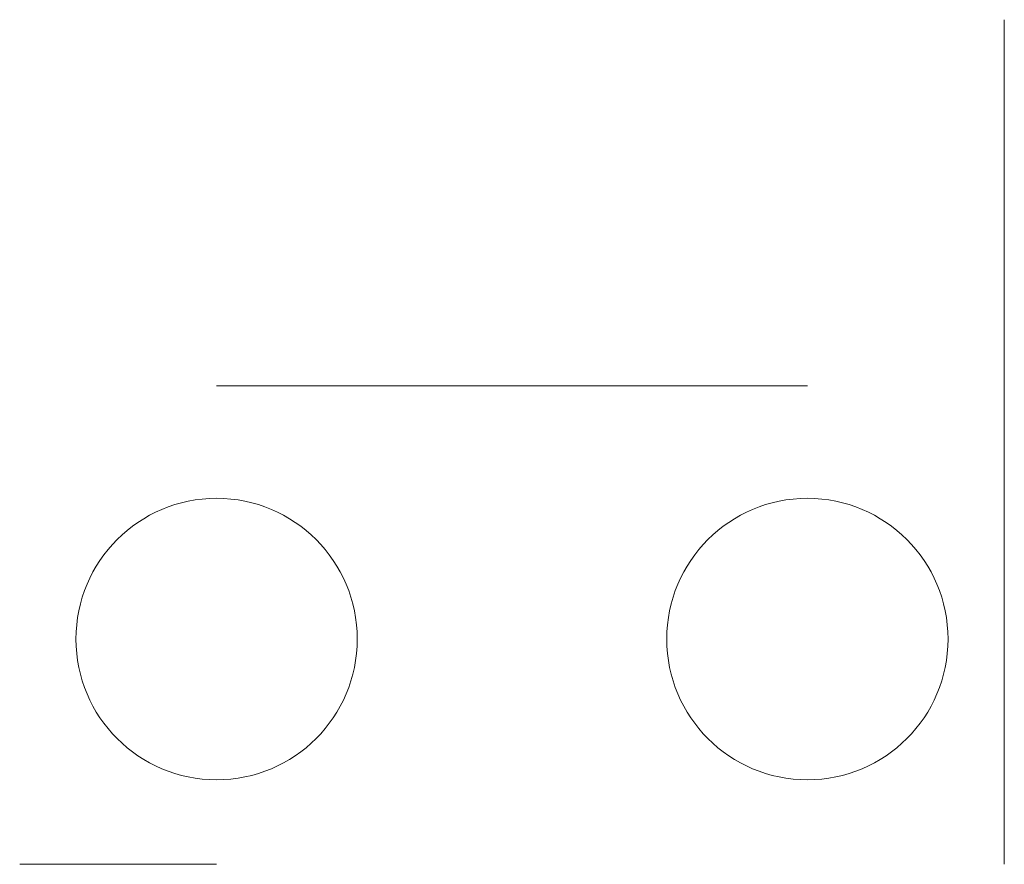
# Model space of a CAD drawing. Units: millimetres. Extents: x -35 to 77, y -482 to 0.
# Tile 1 of 2: x -35 to 0, y -482 to -452. Entities that reach past the tile are written whole.
import ezdxf

# ---------------------------------------------------------------- set-up
doc = ezdxf.new("R2010")
doc.units = ezdxf.units.MM
doc.layers.add('M-CONS', color=8, linetype='Continuous', lineweight=13)

msp = doc.modelspace()

# ---------------------------------------------------------------- linework, layer by layer
at = {"layer": 'M-CONS', "extrusion": (-1, 0, 0)}
for p, q in [((0, -452.364, 152.362), (0, -482.364, 152.362)), ((0, -452.364, 222.362), (0, -452.364, 152.362)), ((0, -460.364, 227.362), (0, -457.364, 227.362)), ((0, -482.364, 162.362), (0, -459.364, 162.362)), ((0, -459.364, 162.362), (0, -459.364, 207.362)), ((0, -459.364, 207.362), (0, -465.364, 207.362)), ((0, -465.364, 207.362), (0, -465.364, 222.362)), ((-35, -482.364, 162.362), (-28, -482.364, 162.362)), ((0, -482.364, 152.362), (0, -482.364, 162.362))]:
    msp.add_line(p, q, dxfattribs=at)
at = {"layer": 'M-CONS', "extrusion": (0, -1, 0), "elevation": 465.364}
msp.add_lwpolyline([(-23, 219.862, 1), (-23, 209.862), (-12, 209.862, 1), (-12, 219.862)], format="xyb", close=True, dxfattribs=at)
at = {"layer": 'M-CONS'}
for centre in [(-28, -474.364, 162.362), (-7, -474.364, 162.362)]:
    msp.add_circle(centre, 5, dxfattribs=at)
at = {"layer": 'M-CONS', "extrusion": (-1, 0, 0)}
for centre, start, end in [((457.364, 222.362), 90, 180), ((460.364, 222.362), 0, 90)]:
    msp.add_arc(centre, 5, start, end, dxfattribs=at)

doc.saveas('drawing.dxf')
